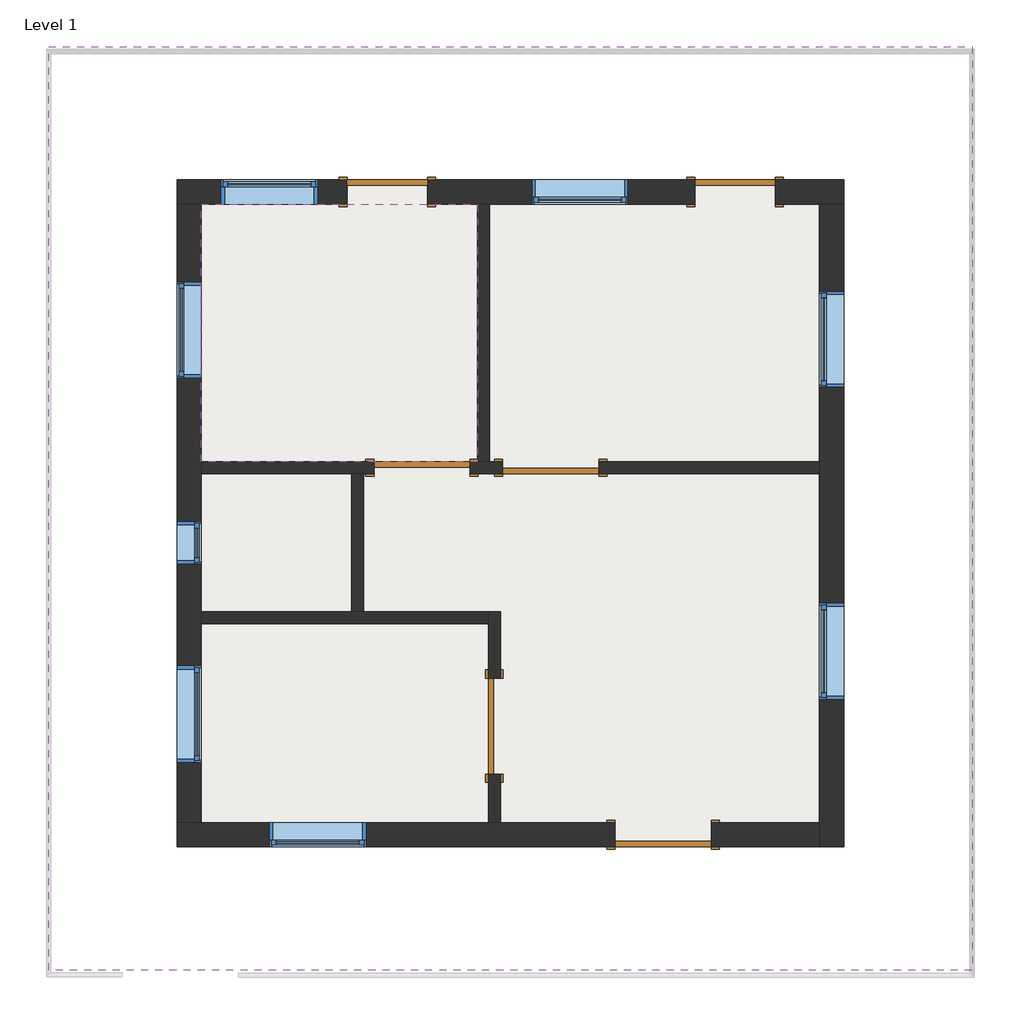
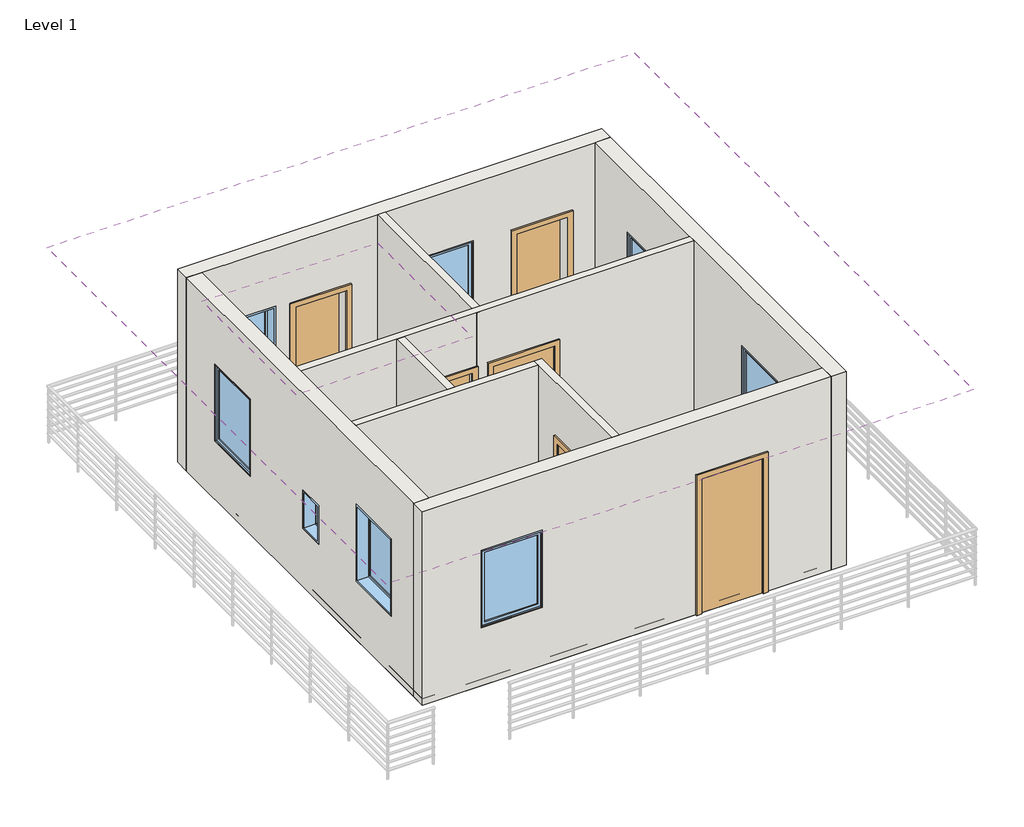
# One storey, part 1 of 2: 9 walls, 8 windows, 6 doors, 2 coverings, 1 slab.
"""IFC4 building model written with IfcOpenShell, lengths in millimetres."""

from ifc_helpers import new_model, si_unit, frame, origin, origin_with_axes, place, context, project, spatial, polyline, outline, extrude, faceted_brep, transform, mapped, element, save
from components import m_single_flush_0762_x_2032mm_ddb9f746, m_single_flush_0915_x_2134mm_2427376d, m_single_flush_0915_x_2134mm_1ddf3370, m_fixed_0406_x_0610mm_6289636b, m_fixed_0915_x_1220mm_b7e646b7

model = new_model("IFC4")

# Units and contexts
model_context = context("Model", 3, world=origin())
ifc_project = project(units=[si_unit("LENGTHUNIT", "METRE", prefix="MILLI")], contexts=[model_context])

# Site, building, storey
site = spatial("IfcSite", under=ifc_project)
building = spatial("IfcBuilding", under=site)
storey = spatial("IfcBuildingStorey", under=building, Name="Level 1", Elevation=0.0)

# Coverings
placement = place(None, origin())
element("IfcCovering", 1, ObjectType="600 x 600mm grid", at=placement, inside=storey, context=model_context, shape_type="SweptSolid", body=[
    extrude(outline(polyline([(-15072.1443193, 2478.2356469), (-12449.5943193, 2478.2356469), (-12449.5943193, 33.8322788), (-15072.1443193, 33.8322788), (-15072.1443193, 2478.2356469)])), frame((0.0, 0.0, 2600.0), z_axis=(0.0, 0.0, 1.0), x_axis=(1.0, 0.0, 0.0)), (0.0, 0.0, 1.0), 101.6),
])
element("IfcCovering", 2, ObjectType="600 x 600mm grid", at=placement, inside=storey, context=model_context, shape_type="SweptSolid", body=[
    extrude(outline(polyline([(-7756.9443193, 3971.7127776), (-7756.9443193, -4791.2872224), (-16519.9443193, -4791.2872224), (-16519.9443193, 3971.7127776), (-7756.9443193, 3971.7127776)])), frame((0.0, 0.0, 3048.0), z_axis=(0.0, 0.0, 1.0), x_axis=(1.0, 0.0, 0.0)), (0.0, 0.0, 1.0), 101.6),
])

# Doors
m_single_flush_0762_x_2032mm_shape = m_single_flush_0762_x_2032mm_ddb9f746(model_context)
element("IfcDoor", 3, ObjectType="M_Single-Flush : 0762 x 2032mm", at=placement, inside=storey, context=model_context, shape_type="MappedRepresentation", body=[
    mapped(m_single_flush_0762_x_2032mm_shape, transform((-13306.8443193, 2592.5356469, 0.0), x_axis=(1.0, 0.0, 0.0), y_axis=(0.0, 1.0, 0.0), z_axis=(0.0, 0.0, 1.0))),
])
element("IfcDoor", 4, ObjectType="M_Single-Flush : 0762 x 2032mm", at=placement, inside=storey, context=model_context, shape_type="MappedRepresentation", body=[
    mapped(m_single_flush_0762_x_2032mm_shape, transform((-10004.8443193, 2592.5356469, 0.0), x_axis=(1.0, 0.0, 0.0), y_axis=(0.0, 1.0, 0.0), z_axis=(0.0, 0.0, 1.0))),
])
m_single_flush_0915_x_2134mm_shape = m_single_flush_0915_x_2134mm_2427376d(model_context)
element("IfcDoor", 5, ObjectType="M_Single-Flush : 0915 x 2134mm", at=placement, inside=storey, context=model_context, shape_type="MappedRepresentation", body=[
    mapped(m_single_flush_0915_x_2134mm_shape, transform((-11757.4443193, -23.3177212, 0.0), x_axis=(-1.0, 0.0, 0.0), y_axis=(0.0, -1.0, 0.0), z_axis=(0.0, 0.0, 1.0))),
])
element("IfcDoor", 6, ObjectType="M_Single-Flush : 0915 x 2134mm", at=placement, inside=storey, context=model_context, shape_type="MappedRepresentation", body=[
    mapped(m_single_flush_0915_x_2134mm_shape, transform((-12976.6443193, -23.3177212, 0.0), x_axis=(1.0, 0.0, 0.0), y_axis=(0.0, 1.0, 0.0), z_axis=(0.0, 0.0, 1.0))),
])
element("IfcDoor", 7, ObjectType="M_Single-Flush : 0915 x 2134mm", at=placement, inside=storey, context=model_context, shape_type="MappedRepresentation", body=[
    mapped(m_single_flush_0915_x_2134mm_shape, transform((-12290.8443193, -2474.5910372, 0.0), x_axis=(0.0, 1.0, 0.0), y_axis=(-1.0, 0.0, 0.0), z_axis=(0.0, 0.0, 1.0))),
])
m_single_flush_0915_x_2134mm_2_shape = m_single_flush_0915_x_2134mm_1ddf3370(model_context)
element("IfcDoor", 8, ObjectType="M_Single-Flush : 0915 x 2134mm", at=placement, inside=storey, context=model_context, shape_type="MappedRepresentation", body=[
    mapped(m_single_flush_0915_x_2134mm_2_shape, transform((-10690.6443193, -3503.4643531, 0.0), x_axis=(-1.0, 0.0, 0.0), y_axis=(0.0, -1.0, 0.0), z_axis=(0.0, 0.0, 1.0))),
])

# Slab
element("IfcSlab", 9, ObjectType="FLOOR 4\"", at=placement, inside=storey, context=model_context, shape_type="SweptSolid", body=[
    extrude(outline(polyline([(-8976.1443193, 2706.8356469), (-8976.1443193, -3617.7643531), (-15300.7443193, -3617.7643531), (-15300.7443193, 2706.8356469), (-8976.1443193, 2706.8356469)])), origin_with_axes(), (0.0, 0.0, 1.0), 101.6),
])

# Walls
element("IfcWall", 10, ObjectType="4,5\"", at=placement, inside=storey, context=model_context, shape_type="Brep", body=[
    faceted_brep([(-12233.6943193, -2017.0910372, 2134.0), (-12233.6943193, -2017.0910372, 0.0), (-12233.6943193, -1388.5677212, 0.0), (-12233.6943193, -1388.5677212, 3048.0), (-12233.6943193, -3389.1643531, 3048.0), (-12233.6943193, -3389.1643531, 0.0), (-12233.6943193, -2932.0910372, 0.0), (-12233.6943193, -2932.0910372, 2134.0), (-12347.9943193, -1388.5677212, 0.0), (-12347.9943193, -1502.8677212, 0.0), (-12347.9943193, -2017.0910372, 0.0), (-12347.9943193, -2017.0910372, 2134.0), (-12347.9943193, -2932.0910372, 2134.0), (-12347.9943193, -2932.0910372, 0.0), (-12347.9943193, -3389.1643531, 0.0), (-12347.9943193, -3389.1643531, 3048.0), (-12347.9943193, -1502.8677212, 3048.0), (-12347.9943193, -1388.5677212, 3048.0)], [[[0, 1, 2, 3, 4, 5, 6, 7]], [[8, 9, 10, 11, 12, 13, 14, 15, 16, 17]], [[6, 5, 14, 13]], [[2, 1, 10, 9, 8]], [[4, 3, 17, 16, 15]], [[5, 4, 15, 14]], [[3, 2, 8, 17]], [[11, 10, 1, 0]], [[12, 11, 0, 7]], [[13, 12, 7, 6]]]),
])
element("IfcWall", 11, ObjectType="4,5\"", at=placement, inside=storey, context=model_context, shape_type="Brep", body=[
    faceted_brep([(-12519.1443193, -80.4677212, 2134.0), (-12519.1443193, -80.4677212, 0.0), (-12449.5943193, -80.4677212, 0.0), (-12335.2943193, -80.4677212, 0.0), (-12214.9443193, -80.4677212, 0.0), (-12214.9443193, -80.4677212, 2134.0), (-11299.9443193, -80.4677212, 2134.0), (-11299.9443193, -80.4677212, 0.0), (-9204.7443193, -80.4677212, 0.0), (-9204.7443193, -80.4677212, 3048.0), (-12335.2943193, -80.4677212, 3048.0), (-12449.5943193, -80.4677212, 3048.0), (-13529.0943193, -80.4677212, 3048.0), (-13643.3943193, -80.4677212, 3048.0), (-15072.1443193, -80.4677212, 3048.0), (-15072.1443193, -80.4677212, 0.0), (-13643.3943193, -80.4677212, 0.0), (-13529.0943193, -80.4677212, 0.0), (-13434.1443193, -80.4677212, 0.0), (-13434.1443193, -80.4677212, 2134.0), (-12214.9443193, 33.8322788, 0.0), (-12335.2943193, 33.8322788, 0.0), (-12449.5943193, 33.8322788, 0.0), (-12519.1443193, 33.8322788, 0.0), (-12519.1443193, 33.8322788, 2134.0), (-13434.1443193, 33.8322788, 2134.0), (-13434.1443193, 33.8322788, 0.0), (-15072.1443193, 33.8322788, 0.0), (-15072.1443193, 33.8322788, 3048.0), (-12449.5943193, 33.8322788, 3048.0), (-12335.2943193, 33.8322788, 3048.0), (-9204.7443193, 33.8322788, 3048.0), (-9204.7443193, 33.8322788, 0.0), (-11299.9443193, 33.8322788, 0.0), (-11299.9443193, 33.8322788, 2134.0), (-12214.9443193, 33.8322788, 2134.0)], [[[0, 1, 2, 3, 4, 5, 6, 7, 8, 9, 10, 11, 12, 13, 14, 15, 16, 17, 18, 19]], [[20, 21, 22, 23, 24, 25, 26, 27, 28, 29, 30, 31, 32, 33, 34, 35]], [[33, 32, 8, 7]], [[18, 17, 16, 15, 27, 26]], [[4, 3, 2, 1, 23, 22, 21, 20]], [[14, 13, 12, 11, 10, 9, 31, 30, 29, 28]], [[9, 8, 32, 31]], [[15, 14, 28, 27]], [[5, 4, 20, 35]], [[6, 5, 35, 34]], [[7, 6, 34, 33]], [[24, 23, 1, 0]], [[25, 24, 0, 19]], [[26, 25, 19, 18]]]),
])
element("IfcWall", 12, ObjectType="4,5\"", at=placement, inside=storey, context=model_context, shape_type="SweptSolid", body=[
    extrude(outline(polyline([(-13529.0943193, -80.4677212), (-13529.0943193, -1388.5677212), (-13643.3943193, -1388.5677212), (-13643.3943193, -80.4677212), (-13529.0943193, -80.4677212)])), origin_with_axes(), (0.0, 0.0, 1.0), 3048.0),
])
element("IfcWall", 13, ObjectType="4,5\"", at=placement, inside=storey, context=model_context, shape_type="Brep", body=[
    faceted_brep([(-15072.1443193, -1502.8677212, 0.0), (-12347.9943193, -1502.8677212, 0.0), (-12347.9943193, -1502.8677212, 3048.0), (-15072.1443193, -1502.8677212, 3048.0), (-15072.1443193, -1388.5677212, 0.0), (-15072.1443193, -1388.5677212, 3048.0), (-13643.3943193, -1388.5677212, 3048.0), (-13529.0943193, -1388.5677212, 3048.0), (-12347.9943193, -1388.5677212, 3048.0), (-12347.9943193, -1388.5677212, 0.0), (-13529.0943193, -1388.5677212, 0.0), (-13643.3943193, -1388.5677212, 0.0)], [[[0, 1, 2, 3]], [[4, 5, 6, 7, 8, 9, 10, 11]], [[1, 0, 4, 11, 10, 9]], [[3, 2, 8, 7, 6, 5]], [[0, 3, 5, 4]], [[2, 1, 9, 8]]]),
])
element("IfcWall", 14, ObjectType="4,5\"", at=placement, inside=storey, context=model_context, shape_type="SweptSolid", body=[
    extrude(outline(polyline([(-12335.2943193, -80.8143531), (-12449.5943193, -80.8143531), (-12449.5943193, -80.4677212), (-12335.2943193, -80.4677212), (-12335.2943193, -80.8143531)])), origin_with_axes(), (0.0, 0.0, 1.0), 3048.0),
    extrude(outline(polyline([(-12449.5943193, 2478.2356469), (-12335.2943193, 2478.2356469), (-12335.2943193, 33.8322788), (-12449.5943193, 33.8322788), (-12449.5943193, 2478.2356469)])), origin_with_axes(), (0.0, 0.0, 1.0), 3048.0),
])
element("IfcWall", 15, ObjectType="9\"", at=placement, inside=storey, context=model_context, shape_type="Brep", body=[
    faceted_brep([(-9623.8443193, 2478.2356469, 2032.0), (-9623.8443193, 2478.2356469, 0.0), (-9204.7443193, 2478.2356469, 0.0), (-8976.1443193, 2478.2356469, 0.0), (-8976.1443193, 2478.2356469, 3048.0), (-9204.7443193, 2478.2356469, 3048.0), (-12335.2943193, 2478.2356469, 3048.0), (-12449.5943193, 2478.2356469, 3048.0), (-15072.1443193, 2478.2356469, 3048.0), (-15300.7443193, 2478.2356469, 3048.0), (-15300.7443193, 2478.2356469, 0.0), (-15072.1443193, 2478.2356469, 0.0), (-13687.8443193, 2478.2356469, 0.0), (-13687.8443193, 2478.2356469, 2032.0), (-12925.8443193, 2478.2356469, 2032.0), (-12925.8443193, 2478.2356469, 0.0), (-12449.5943193, 2478.2356469, 0.0), (-12335.2943193, 2478.2356469, 0.0), (-10385.8443193, 2478.2356469, 0.0), (-10385.8443193, 2478.2356469, 2032.0), (-11020.5443193, 2478.2356469, 915.0), (-11935.5443193, 2478.2356469, 915.0), (-11935.5443193, 2478.2356469, 2135.0), (-11020.5443193, 2478.2356469, 2135.0), (-14881.9443193, 2478.2356469, 915.0), (-14881.9443193, 2478.2356469, 2135.0), (-13966.9443193, 2478.2356469, 2135.0), (-13966.9443193, 2478.2356469, 915.0), (-8976.1443193, 2706.8356469, 0.0), (-9623.8443193, 2706.8356469, 0.0), (-9623.8443193, 2706.8356469, 2032.0), (-10385.8443193, 2706.8356469, 2032.0), (-10385.8443193, 2706.8356469, 0.0), (-12925.8443193, 2706.8356469, 0.0), (-12925.8443193, 2706.8356469, 2032.0), (-13687.8443193, 2706.8356469, 2032.0), (-13687.8443193, 2706.8356469, 0.0), (-15300.7443193, 2706.8356469, 0.0), (-15300.7443193, 2706.8356469, 3048.0), (-8976.1443193, 2706.8356469, 3048.0), (-11020.5443193, 2706.8356469, 915.0), (-11020.5443193, 2706.8356469, 2135.0), (-11935.5443193, 2706.8356469, 2135.0), (-11935.5443193, 2706.8356469, 915.0), (-14881.9443193, 2706.8356469, 915.0), (-13966.9443193, 2706.8356469, 915.0), (-13966.9443193, 2706.8356469, 2135.0), (-14881.9443193, 2706.8356469, 2135.0)], [[[0, 1, 2, 3, 4, 5, 6, 7, 8, 9, 10, 11, 12, 13, 14, 15, 16, 17, 18, 19], [20, 21, 22, 23], [24, 25, 26, 27]], [[28, 29, 30, 31, 32, 33, 34, 35, 36, 37, 38, 39], [40, 41, 42, 43], [44, 45, 46, 47]], [[12, 11, 10, 37, 36]], [[3, 2, 1, 29, 28]], [[18, 17, 16, 15, 33, 32]], [[9, 8, 7, 6, 5, 4, 39, 38]], [[4, 3, 28, 39]], [[10, 9, 38, 37]], [[34, 33, 15, 14]], [[35, 34, 14, 13]], [[36, 35, 13, 12]], [[30, 29, 1, 0]], [[31, 30, 0, 19]], [[32, 31, 19, 18]], [[41, 40, 20, 23]], [[42, 41, 23, 22]], [[43, 42, 22, 21]], [[40, 43, 21, 20]], [[25, 24, 44, 47]], [[26, 25, 47, 46]], [[27, 26, 46, 45]], [[24, 27, 45, 44]]]),
])
element("IfcWall", 16, ObjectType="9\"", at=placement, inside=storey, context=model_context, shape_type="Brep", body=[
    faceted_brep([(-9204.7443193, 2478.2356469, 0.0), (-9204.7443193, 33.8322788, 0.0), (-9204.7443193, -80.4677212, 0.0), (-9204.7443193, -3389.1643531, 0.0), (-9204.7443193, -3617.7643531, 0.0), (-9204.7443193, -3617.7643531, 3048.0), (-9204.7443193, -3389.1643531, 3048.0), (-9204.7443193, -80.4677212, 3048.0), (-9204.7443193, 33.8322788, 3048.0), (-9204.7443193, 2478.2356469, 3048.0), (-9204.7443193, 738.3822788, 915.0), (-9204.7443193, 1653.3822788, 915.0), (-9204.7443193, 1653.3822788, 2135.0), (-9204.7443193, 738.3822788, 2135.0), (-9204.7443193, -2220.8910372, 915.0), (-9204.7443193, -1305.8910372, 915.0), (-9204.7443193, -1305.8910372, 2135.0), (-9204.7443193, -2220.8910372, 2135.0), (-8976.1443193, 2478.2356469, 0.0), (-8976.1443193, 2478.2356469, 3048.0), (-8976.1443193, -3617.7643531, 3048.0), (-8976.1443193, -3617.7643531, 0.0), (-8976.1443193, 738.3822788, 915.0), (-8976.1443193, 738.3822788, 2135.0), (-8976.1443193, 1653.3822788, 2135.0), (-8976.1443193, 1653.3822788, 915.0), (-8976.1443193, -2220.8910372, 915.0), (-8976.1443193, -2220.8910372, 2135.0), (-8976.1443193, -1305.8910372, 2135.0), (-8976.1443193, -1305.8910372, 915.0)], [[[0, 1, 2, 3, 4, 5, 6, 7, 8, 9], [10, 11, 12, 13], [14, 15, 16, 17]], [[18, 19, 20, 21], [22, 23, 24, 25], [26, 27, 28, 29]], [[4, 3, 2, 1, 0, 18, 21]], [[9, 8, 7, 6, 5, 20, 19]], [[0, 9, 19, 18]], [[5, 4, 21, 20]], [[23, 22, 10, 13]], [[24, 23, 13, 12]], [[25, 24, 12, 11]], [[22, 25, 11, 10]], [[27, 26, 14, 17]], [[28, 27, 17, 16]], [[29, 28, 16, 15]], [[26, 29, 15, 14]]]),
])
element("IfcWall", 17, ObjectType="9\"", at=placement, inside=storey, context=model_context, shape_type="Brep", body=[
    faceted_brep([(-11148.1443193, -3389.1643531, 2134.0), (-11148.1443193, -3389.1643531, 0.0), (-12233.6943193, -3389.1643531, 0.0), (-12347.9943193, -3389.1643531, 0.0), (-15072.1443193, -3389.1643531, 0.0), (-15300.7443193, -3389.1643531, 0.0), (-15300.7443193, -3389.1643531, 3048.0), (-15072.1443193, -3389.1643531, 3048.0), (-12347.9943193, -3389.1643531, 3048.0), (-12233.6943193, -3389.1643531, 3048.0), (-9204.7443193, -3389.1643531, 3048.0), (-9204.7443193, -3389.1643531, 0.0), (-10233.1443193, -3389.1643531, 0.0), (-10233.1443193, -3389.1643531, 2134.0), (-13509.7443193, -3389.1643531, 915.0), (-13509.7443193, -3389.1643531, 2135.0), (-14424.7443193, -3389.1643531, 2135.0), (-14424.7443193, -3389.1643531, 915.0), (-15300.7443193, -3617.7643531, 0.0), (-11148.1443193, -3617.7643531, 0.0), (-11148.1443193, -3617.7643531, 2134.0), (-10233.1443193, -3617.7643531, 2134.0), (-10233.1443193, -3617.7643531, 0.0), (-9204.7443193, -3617.7643531, 0.0), (-9204.7443193, -3617.7643531, 3048.0), (-15300.7443193, -3617.7643531, 3048.0), (-13509.7443193, -3617.7643531, 915.0), (-14424.7443193, -3617.7643531, 915.0), (-14424.7443193, -3617.7643531, 2135.0), (-13509.7443193, -3617.7643531, 2135.0)], [[[0, 1, 2, 3, 4, 5, 6, 7, 8, 9, 10, 11, 12, 13], [14, 15, 16, 17]], [[18, 19, 20, 21, 22, 23, 24, 25], [26, 27, 28, 29]], [[12, 11, 23, 22]], [[5, 4, 3, 2, 1, 19, 18]], [[10, 9, 8, 7, 6, 25, 24]], [[11, 10, 24, 23]], [[6, 5, 18, 25]], [[20, 19, 1, 0]], [[21, 20, 0, 13]], [[22, 21, 13, 12]], [[15, 14, 26, 29]], [[16, 15, 29, 28]], [[17, 16, 28, 27]], [[14, 17, 27, 26]]]),
])
element("IfcWall", 18, ObjectType="9\"", at=placement, inside=storey, context=model_context, shape_type="Brep", body=[
    faceted_brep([(-15072.1443193, -3389.1643531, 0.0), (-15072.1443193, -1502.8677212, 0.0), (-15072.1443193, -1388.5677212, 0.0), (-15072.1443193, -80.4677212, 0.0), (-15072.1443193, 33.8322788, 0.0), (-15072.1443193, 2478.2356469, 0.0), (-15072.1443193, 2478.2356469, 3048.0), (-15072.1443193, 33.8322788, 3048.0), (-15072.1443193, -80.4677212, 3048.0), (-15072.1443193, -1388.5677212, 3048.0), (-15072.1443193, -1502.8677212, 3048.0), (-15072.1443193, -3389.1643531, 3048.0), (-15072.1443193, 827.1089628, 915.0), (-15072.1443193, 827.1089628, 2135.0), (-15072.1443193, 1742.1089628, 2135.0), (-15072.1443193, 1742.1089628, 915.0), (-15072.1443193, -1902.6177212, 915.0), (-15072.1443193, -2817.6177212, 915.0), (-15072.1443193, -2817.6177212, 2135.0), (-15072.1443193, -1902.6177212, 2135.0), (-15072.1443193, -531.5177212, 915.0), (-15072.1443193, -937.5177212, 915.0), (-15072.1443193, -937.5177212, 1525.0), (-15072.1443193, -531.5177212, 1525.0), (-15300.7443193, -3389.1643531, 0.0), (-15300.7443193, -3389.1643531, 3048.0), (-15300.7443193, 2478.2356469, 3048.0), (-15300.7443193, 2478.2356469, 0.0), (-15300.7443193, 827.1089628, 915.0), (-15300.7443193, 1742.1089628, 915.0), (-15300.7443193, 1742.1089628, 2135.0), (-15300.7443193, 827.1089628, 2135.0), (-15300.7443193, -1902.6177212, 915.0), (-15300.7443193, -1902.6177212, 2135.0), (-15300.7443193, -2817.6177212, 2135.0), (-15300.7443193, -2817.6177212, 915.0), (-15300.7443193, -531.5177212, 915.0), (-15300.7443193, -531.5177212, 1525.0), (-15300.7443193, -937.5177212, 1525.0), (-15300.7443193, -937.5177212, 915.0)], [[[0, 1, 2, 3, 4, 5, 6, 7, 8, 9, 10, 11], [12, 13, 14, 15], [16, 17, 18, 19], [20, 21, 22, 23]], [[24, 25, 26, 27], [28, 29, 30, 31], [32, 33, 34, 35], [36, 37, 38, 39]], [[5, 4, 3, 2, 1, 0, 24, 27]], [[11, 10, 9, 8, 7, 6, 26, 25]], [[6, 5, 27, 26]], [[0, 11, 25, 24]], [[13, 12, 28, 31]], [[14, 13, 31, 30]], [[15, 14, 30, 29]], [[12, 15, 29, 28]], [[33, 32, 16, 19]], [[34, 33, 19, 18]], [[35, 34, 18, 17]], [[32, 35, 17, 16]], [[37, 36, 20, 23]], [[38, 37, 23, 22]], [[39, 38, 22, 21]], [[36, 39, 21, 20]]]),
])

# Windows
m_fixed_0406_x_0610mm_shape = m_fixed_0406_x_0610mm_6289636b(model_context)
element("IfcWindow", 19, ObjectType="M_Fixed : 0406 x 0610mm", at=placement, inside=storey, context=model_context, shape_type="MappedRepresentation", body=[
    mapped(m_fixed_0406_x_0610mm_shape, transform((-15199.4443193, -734.5177212, 0.0), x_axis=(0.0, -1.0, 0.0), y_axis=(1.0, 0.0, 0.0), z_axis=(0.0, 0.0, 1.0))),
])
m_fixed_0915_x_1220mm_shape = m_fixed_0915_x_1220mm_b7e646b7(model_context)
element("IfcWindow", 20, ObjectType="M_Fixed : 0915 x 1220mm", at=placement, inside=storey, context=model_context, shape_type="MappedRepresentation", body=[
    mapped(m_fixed_0915_x_1220mm_shape, transform((-15173.4443193, 1284.6089628, 0.0), x_axis=(0.0, 1.0, 0.0), y_axis=(-1.0, 0.0, 0.0), z_axis=(0.0, 0.0, 1.0))),
])
element("IfcWindow", 21, ObjectType="M_Fixed : 0915 x 1220mm", at=placement, inside=storey, context=model_context, shape_type="MappedRepresentation", body=[
    mapped(m_fixed_0915_x_1220mm_shape, transform((-9077.4443193, 1195.8822788, 0.0), x_axis=(0.0, 1.0, 0.0), y_axis=(-1.0, 0.0, 0.0), z_axis=(0.0, 0.0, 1.0))),
])
element("IfcWindow", 22, ObjectType="M_Fixed : 0915 x 1220mm", at=placement, inside=storey, context=model_context, shape_type="MappedRepresentation", body=[
    mapped(m_fixed_0915_x_1220mm_shape, transform((-9077.4443193, -1763.3910372, 0.0), x_axis=(0.0, 1.0, 0.0), y_axis=(-1.0, 0.0, 0.0), z_axis=(0.0, 0.0, 1.0))),
])
element("IfcWindow", 23, ObjectType="M_Fixed : 0915 x 1220mm", at=placement, inside=storey, context=model_context, shape_type="MappedRepresentation", body=[
    mapped(m_fixed_0915_x_1220mm_shape, transform((-15199.4443193, -2360.1177212, 0.0), x_axis=(0.0, -1.0, 0.0), y_axis=(1.0, 0.0, 0.0), z_axis=(0.0, 0.0, 1.0))),
])
element("IfcWindow", 24, ObjectType="M_Fixed : 0915 x 1220mm", at=placement, inside=storey, context=model_context, shape_type="MappedRepresentation", body=[
    mapped(m_fixed_0915_x_1220mm_shape, transform((-11478.0443193, 2605.5356469, 0.0), x_axis=(-1.0, 0.0, 0.0), y_axis=(0.0, -1.0, 0.0), z_axis=(0.0, 0.0, 1.0))),
])
element("IfcWindow", 25, ObjectType="M_Fixed : 0915 x 1220mm", at=placement, inside=storey, context=model_context, shape_type="MappedRepresentation", body=[
    mapped(m_fixed_0915_x_1220mm_shape, transform((-14424.4443193, 2579.5356469, 0.0), x_axis=(1.0, 0.0, 0.0), y_axis=(0.0, 1.0, 0.0), z_axis=(0.0, 0.0, 1.0))),
])
element("IfcWindow", 26, ObjectType="M_Fixed : 0915 x 1220mm", at=placement, inside=storey, context=model_context, shape_type="MappedRepresentation", body=[
    mapped(m_fixed_0915_x_1220mm_shape, transform((-13967.2443193, -3490.4643531, 0.0), x_axis=(-1.0, 0.0, 0.0), y_axis=(0.0, -1.0, 0.0), z_axis=(0.0, 0.0, 1.0))),
])

save(model, "model.ifc")

# Revit data of these elements
# Type "600 x 600mm grid"
#   built-in parameter 1002203 = 1 (stored number, unit not read)
#   built-in parameter 1002202 = 1 (stored number, unit not read)
#   Layers, outside or top first: 50.8 mm "Default" (function 1); 50.8 mm "Ceiling Tile 600 x 600" (function 5)
# Type "M_Single-Flush : 0762 x 2032mm"
#   Type Mark = "19"
#   Thickness = 51 mm
#   Height = 2032 mm
#   Trim Projection Ext = 25 mm
#   Trim Projection Int = 25 mm
#   Trim Width = 76 mm
#   Width = 762 mm
#   Door Material = Door - Panel
#   Frame Material = Door - Frame
#   Function = (empty or 0)
#   Wall Closure = (empty or 0)
# Type "M_Single-Flush : 0915 x 2134mm"
#   Type Mark = "15"
#   Thickness = 51 mm
#   Height = 2134 mm
#   Trim Projection Ext = 25 mm
#   Trim Projection Int = 25 mm
#   Trim Width = 76 mm
#   Width = 915 mm
#   Door Material = Door - Panel
#   Frame Material = Door - Frame
#   Function = (empty or 0)
#   Wall Closure = (empty or 0)
# Type "FLOOR 4\""
#   Function = 0
#   Layers, outside or top first: 101.6 mm no material (function 1)
# Type "4,5\""
#   Layers, outside or top first: 114.3 mm no material (function 1)
# Type "9\""
#   Layers, outside or top first: 228.6 mm no material (function 1)
# Type "M_Fixed : 0406 x 0610mm"
#   Type Mark = "10"
#   Height = 610 mm
#   Default Sill Height = 915 mm
#   Width = 406 mm
#   Window Inset = 19 mm
#   Frame Exterior Material = Sash
#   Frame Interior Material = Sash
#   Glass Pane Material = Glass
#   Sash = Sash
#   Wall Closure = (empty or 0)
# Type "M_Fixed : 0915 x 1220mm"
#   Type Mark = "15"
#   Height = 1220 mm
#   Default Sill Height = 915 mm
#   Width = 915 mm
#   Window Inset = 19 mm
#   Frame Exterior Material = Sash
#   Frame Interior Material = Sash
#   Glass Pane Material = Glass
#   Sash = Sash
#   Wall Closure = (empty or 0)
# Element 1 (IfcCovering, "600 x 600mm grid")
#   Height Offset From Level = 2600 mm
#   Phase Created = New Construction
#   Materials on its faces: "Ceiling Tile 600 x 600", "Default"
# Element 2 (IfcCovering, "600 x 600mm grid")
#   Height Offset From Level = 3048 mm
#   Phase Created = New Construction
#   Materials on its faces: "Ceiling Tile 600 x 600", "Default"
# Elements 3, 4 (IfcDoor, "M_Single-Flush : 0762 x 2032mm")
#   Phase Created = New Construction
#   Materials on its faces: "Door - Frame", "Door - Panel"
# Elements 5, 6, 7, 8 (IfcDoor, "M_Single-Flush : 0915 x 2134mm")
#   Phase Created = New Construction
#   Materials on its faces: "Door - Frame", "Door - Panel"
# Element 9 (IfcSlab, "FLOOR 4\"")
#   Height Offset From Level = 101.6 mm
#   Phase Created = New Construction
#   Materials on its faces: "Default Roof"
# Elements 10, 11, 12, 13, 14 (IfcWall, "4,5\"")
#   Top Offset = 0 mm
#   Base Offset = 0 mm
#   Unconnected Height = 3048 mm
#   wall height = 3048 mm
#   Phase Created = New Construction
#   Base Constraint = Level 1
#   Materials on its faces: "Default Wall"
# Elements 15, 16, 17, 18 (IfcWall, "9\"")
#   Top Offset = 0 mm
#   Base Offset = 0 mm
#   Unconnected Height = 3048 mm
#   wall height = 3048 mm
#   Phase Created = New Construction
#   Base Constraint = Level 1
#   Materials on its faces: "Default Wall"
# Element 19 (IfcWindow, "M_Fixed : 0406 x 0610mm")
#   Mark = "10"
#   Phase Created = New Construction
#   Materials on its faces: "Sash", "Glass"
# Element 20 (IfcWindow, "M_Fixed : 0915 x 1220mm")
#   Mark = "6"
#   Phase Created = New Construction
#   Materials on its faces: "Sash", "Glass"
# Element 21 (IfcWindow, "M_Fixed : 0915 x 1220mm")
#   Mark = "7"
#   Phase Created = New Construction
#   Materials on its faces: "Sash", "Glass"
# Element 22 (IfcWindow, "M_Fixed : 0915 x 1220mm")
#   Mark = "8"
#   Phase Created = New Construction
#   Materials on its faces: "Sash", "Glass"
# Element 23 (IfcWindow, "M_Fixed : 0915 x 1220mm")
#   Mark = "9"
#   Phase Created = New Construction
#   Materials on its faces: "Sash", "Glass"
# Element 24 (IfcWindow, "M_Fixed : 0915 x 1220mm")
#   Mark = "11"
#   Phase Created = New Construction
#   Materials on its faces: "Sash", "Glass"
# Element 25 (IfcWindow, "M_Fixed : 0915 x 1220mm")
#   Mark = "12"
#   Phase Created = New Construction
#   Materials on its faces: "Sash", "Glass"
# Element 26 (IfcWindow, "M_Fixed : 0915 x 1220mm")
#   Mark = "13"
#   Phase Created = New Construction
#   Materials on its faces: "Sash", "Glass"
# Materials
#   "Default": colour RGB 80 80 80, transparency 0
#   "Ceiling Tile 600 x 600": class "Generic", colour RGB 180 179 177, transparency 0, Description = "Acoustic ceiling tile", Cost = 0
#   "Door - Panel": class "Wood", colour RGB 114 82 51, transparency 0
#   "Door - Frame": colour RGB 153 76 43, transparency 0
#   "Sash": class "Wood", colour RGB 136 99 55, transparency 0
#   "Glass": class "Glass", colour RGB 218 227 224, transparency 0.85, Description = "Soda Lime Glass", Cost = 0
#   "Default Roof": colour RGB 80 80 80, transparency 0
#   "Default Wall": colour RGB 80 80 80, transparency 0
# Room at (-13699.569, 1088.55) mm, phase "New Construction", upper level "Level 1", upper offset 4000.004 mm, lower offset 0 mm
#   Number = "1"
# Room at (-11003.101, 1088.55) mm, phase "New Construction", upper level "Level 1", upper offset 4000.004 mm, lower offset 0 mm
#   Number = "2"
#   Name = "Room"
# Room at (-11139.548, -1599.536) mm, phase "New Construction", upper level "Level 1", upper offset 4000.004 mm, lower offset 0 mm
#   Number = "3"
#   Name = "Room"
# Room at (-13604.109, -2213.544) mm, phase "New Construction", upper level "Level 1", upper offset 4000.004 mm, lower offset 0 mm
#   Number = "4"
#   Name = "Room"
# Room at (-14371.619, -814.97) mm, phase "New Construction", upper level "Level 1", upper offset 4000.004 mm, lower offset 0 mm
#   Number = "5"
#   Name = "Room"
